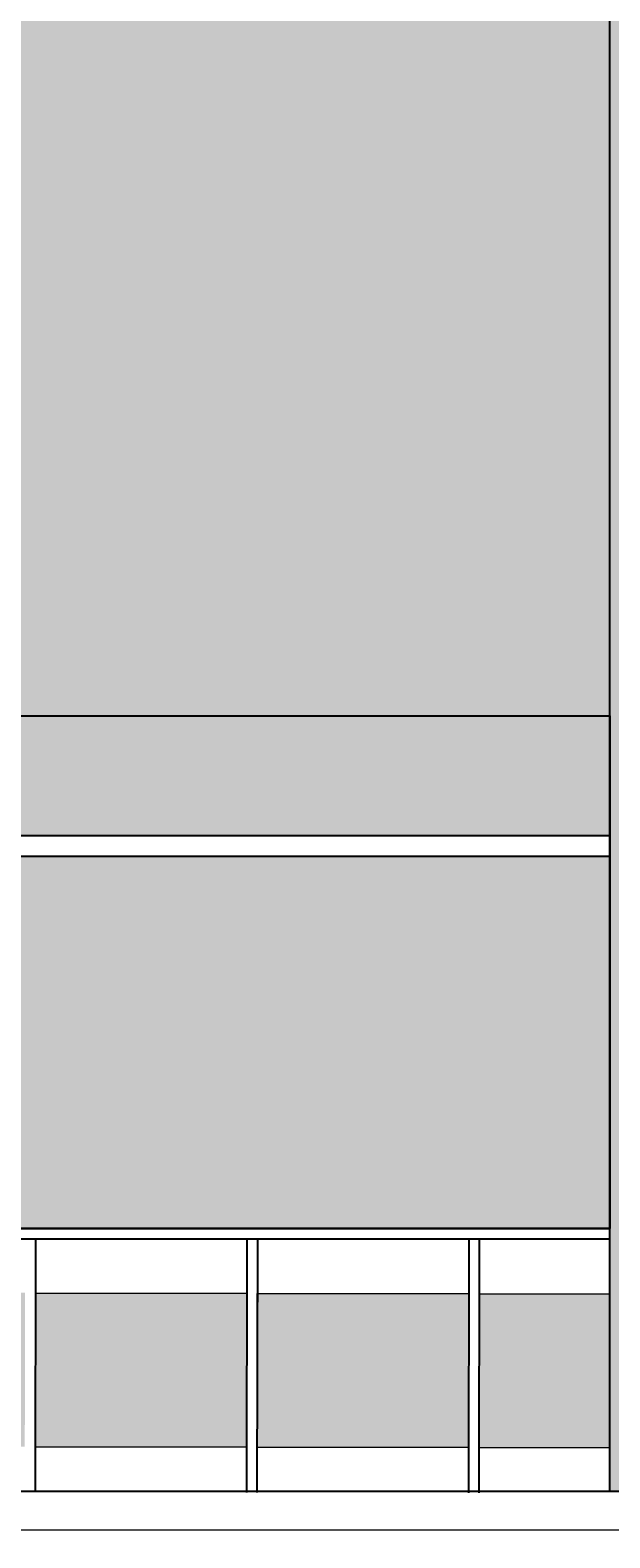
# Model space of a CAD drawing. Units: inches. Extents: x 36 to 594, y 79 to 831.
# Tile 19 of 30: x 286 to 342, y 446 to 590. Entities that reach past the tile are written whole.
import ezdxf

# ---------------------------------------------------------------- set-up
doc = ezdxf.new("R2010")
doc.units = ezdxf.units.IN
doc.header["$MEASUREMENT"] = 0
for name, color, linetype, lineweight in [('A-ANNO-DIMS', 2, 'Continuous', 18), ('A-ELEV', 7, 'Continuous', 25), ('A-ELEV-PATT', 8, 'Continuous', 13), ('A-GLAZ', 4, 'Continuous', 18)]:
    doc.layers.add(name, color=color, linetype=linetype, lineweight=lineweight)
doc.styles.get("Standard").update_dxf_attribs({"font": 'arial.ttf'})
doc.dimstyles.get("Standard").update_dxf_attribs({"dimtxt": 0.8125, "dimasz": 0.18, "dimexe": 0.18, "dimexo": 0.0625, "dimgap": 0.09, "dimtad": 0, "dimtih": 1, "dimtoh": 1, "dimdec": 4, "dimzin": 0, "dimdsep": 46, "dimlunit": 4, "dimtxsty": 'Standard', "dimcen": 0.09, "dimadec": 0, "dimazin": 0, "dimtfac": 1, "dimtdec": 4, "dimtofl": 0, "dimtmove": 0, "dimatfit": 3, "dimfxl": 1, "dimtolj": 1, "dimtzin": 0, "dimarcsym": 0})

# ---------------------------------------------------------------- blocks, each defined once
blk = doc.blocks.new('GLAZ-PANEL')
blk.add_lwpolyline([(0, 14.77), (20.28, 14.77), (20.28, 0), (0, 0)], close=True)
blk = doc.blocks.new('*D95')
at = {"layer": 'A-ANNO-DIMS', "color": 0, "lineweight": -2, "transparency": 16777216}
for p, q in [((260.51, 524.67), (260.51, 830.73)), ((260.69, 830.55), (299.71, 830.55)), ((341.66, 830.55), (302.63, 830.55)), ((341.84, 524.67), (341.84, 830.73))]:
    blk.add_line(p, q, dxfattribs=at)
at = {"layer": 'A-ANNO-DIMS', "color": 0, "transparency": 16777216}
for points in [[(260.69, 830.58), (260.69, 830.52), (260.51, 830.55)], [(341.66, 830.58), (341.66, 830.52), (341.84, 830.55)]]:
    blk.add_solid(points, dxfattribs=at)
at = {"layer": 'Defpoints', "color": 0, "transparency": 16777216}
for p in [(341.84, 830.55), (260.51, 524.6), (341.84, 524.6)]:
    blk.add_point(p, dxfattribs=at)
at = {"layer": 'A-ANNO-DIMS', "color": 0, "transparency": 16777216, "insert": (301.17, 830.55), "char_height": 0.812, "attachment_point": 5}
blk.add_mtext('\\A1;81.33', dxfattribs=at)
blk = doc.blocks.new('*D107')
at = {"layer": 'A-ANNO-DIMS', "color": 0, "lineweight": -2, "transparency": 16777216}
for p, q in [((269.04, 404.34), (269.04, 830.73)), ((269.22, 830.55), (310.99, 830.55)), ((355.68, 830.55), (313.91, 830.55)), ((355.86, 404.34), (355.86, 830.73))]:
    blk.add_line(p, q, dxfattribs=at)
at = {"layer": 'A-ANNO-DIMS', "color": 0, "transparency": 16777216}
for points in [[(269.22, 830.58), (269.22, 830.52), (269.04, 830.55)], [(355.68, 830.58), (355.68, 830.52), (355.86, 830.55)]]:
    blk.add_solid(points, dxfattribs=at)
at = {"layer": 'Defpoints', "color": 0, "transparency": 16777216}
for p in [(355.86, 830.55), (269.04, 404.27), (355.86, 404.27)]:
    blk.add_point(p, dxfattribs=at)
at = {"layer": 'A-ANNO-DIMS', "color": 0, "transparency": 16777216, "insert": (312.45, 830.55), "char_height": 0.812, "attachment_point": 5}
blk.add_mtext('\\A1;86.82', dxfattribs=at)

msp = doc.modelspace()

# ---------------------------------------------------------------- hatches: boundary and pattern name
at = {"layer": 'A-ELEV-PATT'}
h = msp.add_hatch(color=256, dxfattribs=at)
h.dxf.hatch_style = 1
h.paths.add_polyline_path([(398.0873, 796.0465), (269.3592, 796.0465), (269.3592, 770.1455), (397.8159, 770.1455)])
h.paths.add_polyline_path([(397.7518, 764.0341), (269.3592, 764.0341), (269.3592, 630.0394), (341.8367, 630.0394), (341.8367, 720.595), (335.0881, 728.3699), (329.982, 735.3373), (345.3661, 727.7743), (397.1052, 702.3389)])
h.paths.add_polyline_path([(341.8367, 594.2124), (201.4189, 594.2124), (201.4189, 475.4136), (232.8216, 475.4136), (232.8216, 524.6037), (341.8367, 524.6037)])
h.paths.add_polyline_path([(177.525, 594.2124), (118.7598, 594.2124), (118.7598, 450.2124), (177.525, 450.2124)])
h.paths.add_polyline_path([(424.4958, 594.2124), (365.7306, 594.2124), (365.7306, 450.2124), (424.4958, 450.2124)])
h.paths.add_polyline_path([(241.3553, 404.2737), (355.8569, 404.2737), (355.8569, 355.0836), (424.5492, 355.0836), (424.5492, 425.7333), (118.7598, 426.2844), (118.7598, 355.0836), (241.3553, 355.0836)])
h.paths.add_polyline_path([(448.3898, 306.2124), (217.0273, 306.2124), (217.0273, 142.2124), (254.0293, 142.2124), (254.0293, 150.9347), (254.0293, 286.1802), (401.5491, 286.1802), (401.5491, 150.9347), (401.5491, 142.2124), (448.3898, 142.2124)])
h.paths.add_polyline_path([(448.3898, 142.2124), (401.5491, 142.2124), (217.0273, 142.2124), (217.0273, 114.2124), (448.3898, 114.2124)])
h.paths.add_polyline_path([(217.0273, 306.2124), (174.7353, 306.2124), (94.8658, 306.2124), (94.8658, 162.2124), (103.3368, 162.2124), (103.3368, 264.6224), (103.3368, 286.1802), (217.0273, 286.1802)])
h = msp.add_hatch(color=256, dxfattribs=at)
h.dxf.hatch_style = 1
h.paths.add_polyline_path([(448.3898, 668.2124), (341.8367, 720.595), (341.8367, 594.2124), (341.8367, 450.2124), (365.7306, 450.2124), (365.7306, 594.2124), (424.4958, 594.2124), (424.4958, 450.2124), (448.3898, 450.2124), (448.3898, 594.2124)])
h.paths.add_polyline_path([(378.5958, 653.8563, -1), (413.2033, 653.8563, -1)], flags=16)
h.paths.add_polyline_path([(394.8995, 653.8563), (394.8995, 654.8563), (395.8995, 654.8563), (396.8995, 654.8563), (396.8995, 653.8563), (396.8995, 652.8563), (395.8995, 652.8563), (394.8995, 652.8563)], flags=0)
h.paths.add_polyline_path([(201.4189, 708.8485), (201.4189, 720.595), (94.8658, 668.2124), (94.8658, 644.2124), (94.8658, 596.2124), (94.8658, 594.2124), (94.8658, 450.2124), (118.7598, 450.2124), (118.7598, 594.2124), (177.525, 594.2124), (177.525, 450.2124), (201.4189, 450.2124), (201.4189, 594.2124)])
h.paths.add_polyline_path([(130.1589, 653.7648, -1), (164.7665, 653.7648, -1)], flags=16)
h.paths.add_polyline_path([(148.4627, 652.7648), (147.4627, 652.7648), (146.4627, 652.7648), (146.4627, 653.7648), (146.4627, 654.7648), (147.4627, 654.7648), (148.4627, 654.7648), (148.4627, 653.7648)], flags=0)
h = msp.add_hatch(color=256, dxfattribs=at)
h.dxf.hatch_style = 1
h.set_gradient(color1=(0, 255, 255), color2=(16, 86, 137))
h.paths.add_polyline_path([(341.8367, 524.6037), (260.5056, 524.6037), (260.5056, 513.1224), (341.8367, 513.1224)])
h.paths.add_polyline_path([(341.8367, 511.1224), (260.5056, 511.1224), (260.5056, 475.4136), (341.8367, 475.4136)])
h.paths.add_polyline_path([(258.5056, 524.6037), (232.8216, 524.6037), (232.8216, 513.1224), (258.5056, 513.1224)])
h.paths.add_polyline_path([(355.8569, 404.2737), (269.0393, 404.2737), (269.0393, 392.7924), (355.8569, 392.7924)])
h.paths.add_polyline_path([(267.0393, 404.2737), (241.3553, 404.2737), (241.3553, 392.7924), (267.0393, 392.7924)])
h.paths.add_polyline_path([(355.8569, 390.7924), (269.0393, 390.7924), (269.0393, 355.0836), (355.8569, 355.0836)])
h.paths.add_polyline_path([(399.5491, 284.1802), (256.0293, 284.1802), (256.0293, 271.378), (399.5491, 271.378)])
h.paths.add_polyline_path([(317.3533, 259.1243), (262.3169, 259.1243), (262.3169, 200.6645), (317.3533, 200.6645)])
h.paths.add_polyline_path([(390.386, 259.1243), (335.3496, 259.1243), (335.3496, 200.6645), (390.386, 200.6645)])
h.paths.add_polyline_path([(390.386, 190.7697), (335.3496, 190.7697), (335.3496, 162.9881), (390.386, 162.9881)])
h.paths.add_polyline_path([(317.3533, 190.7697), (262.3169, 190.7697), (262.3169, 162.9881), (317.3533, 162.9881)])
h.paths.add_polyline_path([(215.0273, 262.6224), (158.4069, 262.6224), (158.4069, 181.4195), (215.0273, 181.4195)])
h.paths.add_polyline_path([(215.0273, 284.1802), (105.3368, 284.1802), (105.3368, 266.6224), (215.0273, 266.6224)])
h = msp.add_hatch(color=256, dxfattribs=at)
h.dxf.hatch_style = 1
h.set_gradient(color1=(192, 192, 192), color2=(0, 0, 0))
h.paths.add_polyline_path([(243.19, 469.3251), (222.9132, 469.3251), (222.9132, 454.5571), (243.1634, 454.5571)])
h.paths.add_polyline_path([(264.4667, 469.2868), (244.1899, 469.2868), (244.1899, 454.5188), (264.4401, 454.5188)])
h.paths.add_polyline_path([(285.7435, 469.2484), (265.4667, 469.2484), (265.4667, 454.4804), (285.7168, 454.4804)])
h.paths.add_polyline_path([(307.0202, 469.2101), (286.7434, 469.2101), (286.7434, 454.4421), (306.9936, 454.4421)])
h.paths.add_polyline_path([(328.2969, 469.1717), (308.0201, 469.1717), (308.0201, 454.4037), (328.2703, 454.4037)])
h.paths.add_polyline_path([(341.8367, 469.1334), (329.2969, 469.1334), (329.2969, 454.3654), (341.8367, 454.3654)])
h.paths.add_polyline_path([(221.9133, 469.3635), (201.6365, 469.3635), (201.6365, 454.5955), (221.8866, 454.5955)])
h.paths.add_polyline_path([(145.3401, 349.1868), (125.0633, 349.1868), (125.0633, 334.4189), (145.3134, 334.4189)])
h.paths.add_polyline_path([(166.6168, 349.1485), (146.34, 349.1485), (146.34, 334.3805), (166.5902, 334.3805)])
h.paths.add_polyline_path([(187.8935, 349.1101), (167.6167, 349.1101), (167.6167, 334.3422), (187.8669, 334.3422)])
h.paths.add_polyline_path([(209.1703, 349.0718), (188.8935, 349.0718), (188.8935, 334.3038), (209.1436, 334.3038)])
h.paths.add_polyline_path([(230.447, 349.0335), (210.1702, 349.0335), (210.1702, 334.2655), (230.4204, 334.2655)])
h.paths.add_polyline_path([(251.7237, 348.9951), (231.4469, 348.9951), (231.4469, 334.2271), (251.6971, 334.2271)])
h.paths.add_polyline_path([(273.0005, 348.9568), (252.7236, 348.9568), (252.7236, 334.1888), (272.9738, 334.1888)])
h.paths.add_polyline_path([(294.2772, 348.9184), (274.0004, 348.9184), (274.0004, 334.1504), (294.2506, 334.1504)])
h.paths.add_polyline_path([(315.5539, 348.8801), (295.2771, 348.8801), (295.2771, 334.1121), (315.5273, 334.1121)])
h.paths.add_polyline_path([(336.8306, 348.8417), (316.5538, 348.8417), (316.5538, 334.0737), (336.804, 334.0737)])
h.paths.add_polyline_path([(358.1074, 348.8034), (337.8306, 348.8034), (337.8306, 334.0354), (358.0808, 334.0354)])
h.paths.add_polyline_path([(379.3841, 348.765), (359.1073, 348.765), (359.1073, 333.997), (379.3575, 333.997)])
h.paths.add_polyline_path([(400.6608, 348.7267), (380.384, 348.7267), (380.384, 333.9587), (400.6342, 333.9587)])
h.paths.add_polyline_path([(421.9376, 348.6883), (401.6608, 348.6883), (401.6608, 333.9204), (421.911, 333.9204)])
h.paths.add_polyline_path([(103.3368, 162.2124), (94.8658, 162.2124), (94.8658, 150.2124), (94.8658, 114.2124), (103.3368, 114.2124)])
h.paths.add_polyline_path([(217.0273, 132.2124), (103.3368, 132.2124), (103.3368, 122.2124), (217.0273, 122.2124)])
h.paths.add_polyline_path([(217.0273, 122.2124), (103.3368, 122.2124), (103.3368, 114.2124), (217.0273, 114.2124)])
h.paths.add_polyline_path([(217.0273, 142.2124), (174.7353, 142.2124), (103.3368, 142.2124), (103.3368, 132.2124), (217.0273, 132.2124)])
h.paths.add_polyline_path([(217.0273, 152.2124), (103.3368, 152.2124), (103.3368, 142.2124), (174.7353, 142.2124), (217.0273, 142.2124)])
h.paths.add_polyline_path([(217.0273, 162.2124), (103.3368, 162.2124), (103.3368, 152.2124), (217.0273, 152.2124)])
h = msp.add_hatch(dxfattribs=at)
h.set_pattern_fill('ANSI31', color=256, scale=38, angle=135)
h.paths.add_polyline_path([(448.3898, 450.2124), (94.8658, 450.2124), (94.8658, 306.2124), (174.7353, 306.2124), (448.3898, 306.2124), (448.3898, 367.5118)])
h.paths.add_polyline_path([(424.5492, 425.7333), (424.5492, 329.5325), (118.7598, 330.0836), (118.7598, 354.0836), (118.7598, 426.2844)], flags=16)
h.paths.add_polyline_path([(355.8569, 404.2737), (355.8569, 355.0836), (241.3553, 355.0836), (241.3553, 404.2737)], flags=0)
h.paths.add_polyline_path([(269.0393, 390.7924), (269.0393, 355.0836), (244.8248, 355.0836), (244.8248, 364.0887), (263.8892, 364.0887), (263.8892, 355.0836), (267.0393, 355.0836), (267.0393, 390.7924)], flags=0)
h.paths.add_polyline_path([(303.9765, 436.9126, -1), (313.1496, 436.9126, -1)], flags=16)
h.paths.add_polyline_path([(421.9473, 354.0836), (421.9376, 348.6883), (421.9376, 333.9204), (401.6342, 333.9204), (401.6705, 354.0836), (400.6705, 354.0836), (400.6608, 348.7267), (400.6608, 333.9587), (380.3574, 333.9587), (380.3937, 354.0836), (379.3937, 354.0836), (379.3841, 348.765), (379.3841, 333.997), (359.0807, 333.997), (359.1169, 354.0836), (358.1169, 354.0836), (358.1074, 348.8034), (358.1074, 334.0354), (337.804, 334.0354), (337.8401, 354.0836), (336.8401, 354.0836), (336.8306, 348.8417), (336.8306, 334.0737), (316.5272, 334.0737), (316.5633, 354.0836), (315.5633, 354.0836), (315.5539, 348.8801), (315.5539, 334.1121), (295.2505, 334.1121), (295.2865, 354.0836), (294.2865, 354.0836), (294.2772, 348.9184), (294.2772, 334.1504), (273.9738, 334.1504), (274.0097, 354.0836), (273.0097, 354.0836), (273.0005, 348.9568), (273.0005, 334.1888), (252.697, 334.1888), (252.7329, 354.0836), (251.7329, 354.0836), (251.7237, 348.9951), (251.7237, 334.2271), (231.4203, 334.2271), (231.4561, 354.0836), (230.4561, 354.0836), (230.447, 349.0335), (230.447, 334.2655), (210.1436, 334.2655), (210.1793, 354.0836), (209.1793, 354.0836), (209.1703, 349.0718), (209.1703, 334.3038), (188.8668, 334.3038), (188.9025, 354.0836), (187.9025, 354.0836), (187.8935, 349.1101), (187.8935, 334.3422), (167.5901, 334.3422), (167.6257, 354.0836), (166.6257, 354.0836), (166.6168, 349.1485), (166.6168, 334.3805), (146.3134, 334.3805), (146.3489, 354.0836), (145.3489, 354.0836), (145.3401, 349.1868), (145.3401, 334.4189), (125.0366, 334.4189), (125.0721, 354.0836)], flags=0)
h.paths.add_polyline_path([(266.285, 436.9126, -1), (275.458, 436.9126, -1)], flags=16)
h.paths.add_polyline_path([(367.0204, 316.8739, -1), (357.8474, 316.8739, -1)], flags=16)
h.paths.add_polyline_path([(347.6933, 316.8739, -1), (338.5202, 316.8739, -1)], flags=16)
h.paths.add_polyline_path([(329.574, 316.8739, -1), (320.401, 316.8739, -1)], flags=16)
h.paths.add_polyline_path([(263.8892, 385.1199), (263.8892, 368.1628), (244.8248, 368.1628), (244.8248, 385.1199)], flags=0)
h.paths.add_polyline_path([(216.2543, 436.9126, -1), (225.4274, 436.9126, -1)], flags=16)
h.paths.add_polyline_path([(275.458, 316.8739, -1), (266.285, 316.8739, -1)], flags=16)
h.paths.add_polyline_path([(225.4274, 316.8739, -1), (216.2543, 316.8739, -1)], flags=16)

# ---------------------------------------------------------------- linework, layer by layer
at = {"layer": 'A-ELEV'}
for p, q in [((341.8367, 450.2124), (341.8367, 594.2124)), ((232.8216, 513.1224), (341.8367, 513.1224)), ((232.8216, 511.1224), (341.8367, 511.1224)), ((201.4189, 475.4136), (341.8367, 475.4136)), ((201.4189, 474.4136), (341.8367, 474.4136)), ((286.7528, 474.4136), (286.709, 450.1339)), ((307.0296, 474.4136), (306.9857, 450.0973)), ((308.0296, 474.4136), (307.9857, 450.0955)), ((328.3064, 474.4136), (328.2625, 450.059)), ((329.3064, 474.4136), (329.2625, 450.0572)), ((94.8658, 450.2124), (448.3898, 450.2124))]:
    msp.add_line(p, q, dxfattribs=at)
msp.add_lwpolyline([(232.8216, 524.6037), (341.8367, 524.6037), (341.8367, 475.4136), (232.8216, 475.4136)], close=True, dxfattribs=at)
at = {"layer": 'A-GLAZ'}
msp.add_lwpolyline([(341.8367, 454.3654), (329.2969, 454.3654), (329.2969, 469.1334), (341.8367, 469.1334)], dxfattribs=at)

# ---------------------------------------------------------------- block references
for p in [(286.7431, 454.4422), (308.0199, 454.4039)]:
    msp.add_blockref('GLAZ-PANEL', p, dxfattribs=at)

# ---------------------------------------------------------------- dimensions: what is measured, and where the dimension line sits
at = {"layer": 'A-ANNO-DIMS'}
for base, p1, p2, picture, middle in [((341.8367, 830.5465), (260.5056, 524.6037), (341.8367, 524.6037), '*D95', (301.1711, 830.5465)), ((355.8569, 830.5465), (269.0393, 404.2737), (355.8569, 404.2737), '*D107', (312.4481, 830.5465))]:
    dim = msp.add_linear_dim(base=base, p1=p1, p2=p2, dimstyle='Standard', override={"dimdec": 2, "dimlfac": 1, "dimrnd": 0, "dimzin": 0, "dimdsep": 46, "dimlunit": 2}, dxfattribs=at)
    dim.commit()
    dim.dimension.update_dxf_attribs({"geometry": picture, "text_midpoint": middle})

doc.saveas('drawing.dxf')
